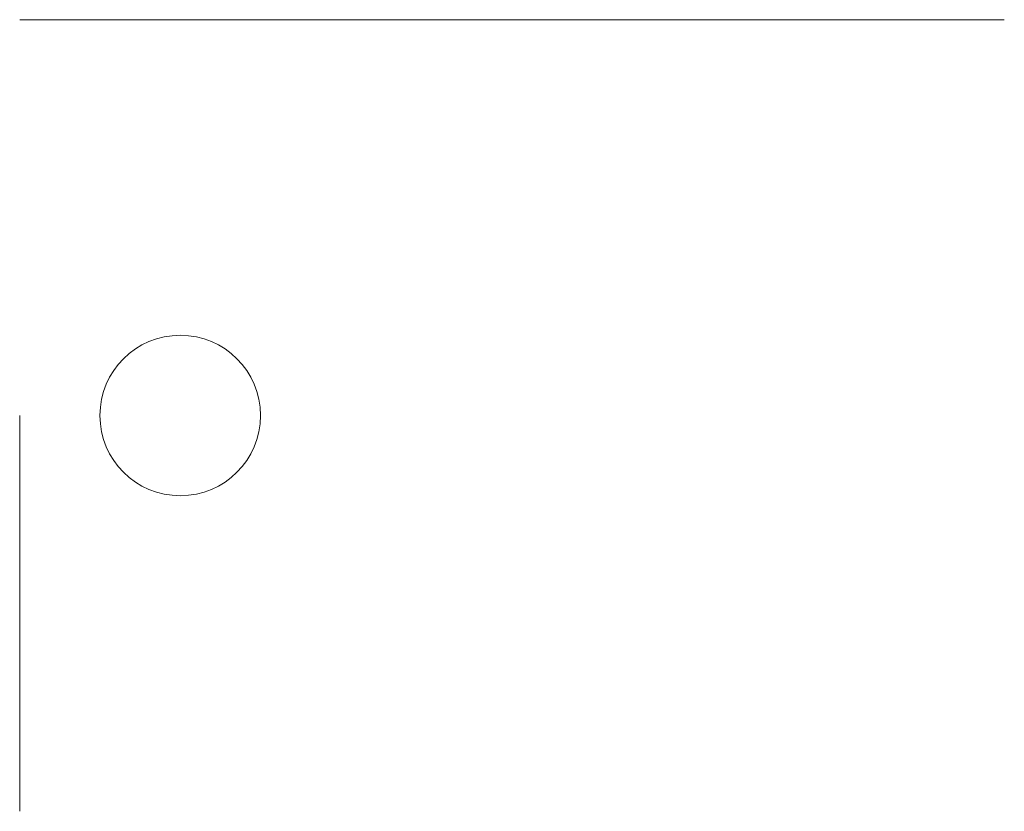
# Model space of a CAD drawing. Units: millimetres. Extents: x 549 to 905, y -110 to 0.
# Tile 1 of 2: x 549 to 641, y -74 to 0. Entities that reach past the tile are written whole.
import ezdxf

# ---------------------------------------------------------------- set-up
doc = ezdxf.new("R2010")
doc.units = ezdxf.units.MM
doc.layers.add('M-CONS', color=8, linetype='Continuous', lineweight=13)

msp = doc.modelspace()

# ---------------------------------------------------------------- linework, layer by layer
at = {"layer": 'M-CONS', "extrusion": (0, -1, 0)}
for p, q in [((549.488, 0, 181.883), (641.488, 0, 181.883)), ((549.488, 0, 181.883), (549.488, 0, 193.883)), ((549.488, 0, 193.883), (629.488, 0, 193.883)), ((629.488, 0, 193.883), (629.488, 0, 268.883))]:
    msp.add_line(p, q, dxfattribs=at)
at = {"layer": 'M-CONS'}
msp.add_line((549.488, -74, 193.883), (549.488, -37, 193.883), dxfattribs=at)
msp.add_circle((564.488, -37, 193.883), 7.5, dxfattribs=at)

doc.saveas('drawing.dxf')
